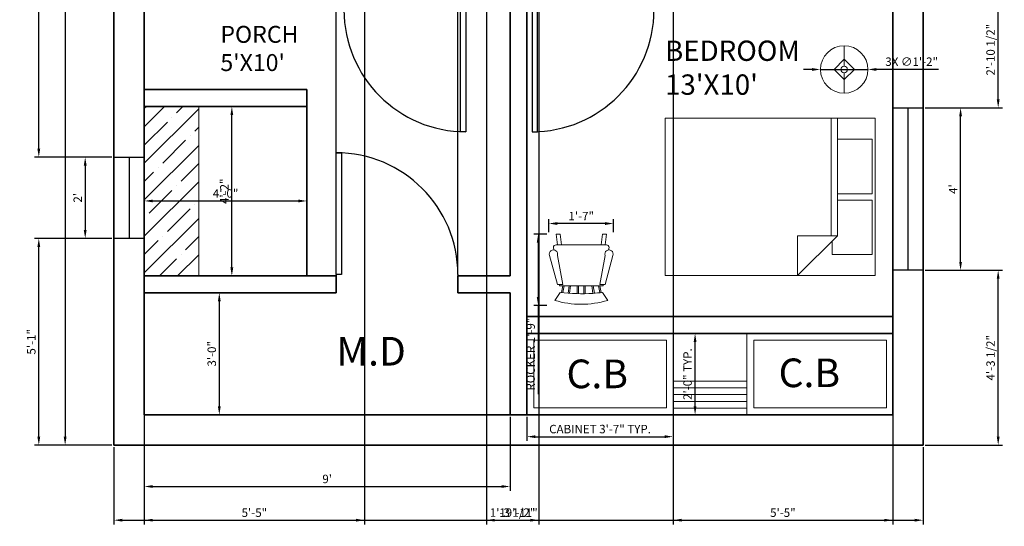
# Model space of a CAD drawing. Units: inches. Extents: x 2459 to 2755, y 1300 to 1776.
# Tile 1 of 4: x 2459 to 2750, y 1300 to 1450. Entities that reach past the tile are written whole.
import ezdxf

# ---------------------------------------------------------------- set-up
doc = ezdxf.new("R2010")
doc.units = ezdxf.units.IN
for name, color, linetype, lineweight in [('A-AREA-IDEN', 3, 'Continuous', 25), ('A-FLOR-CASE', 7, 'Continuous', 20), ('A-FURN-PATT', 8, 'Continuous', 13), ('A-WALL', 7, 'Continuous', 35), ('DIM', 4, 'Continuous', 18), ('DOOR', 20, 'Continuous', 25), ('FURNITURE', 6, 'Continuous', 18), ('TEXT', 3, 'Continuous', 25), ('WIN', 2, 'Continuous', 25)]:
    doc.layers.add(name, color=color, linetype=linetype, lineweight=lineweight)
doc.styles.get("Standard").update_dxf_attribs({"font": 'arial.ttf'})
doc.dimstyles.new('ISO-25', dxfattribs={"dimtxt": 2.5, "dimasz": 2.5, "dimexe": 1.25, "dimexo": 0.625, "dimtad": 1, "dimlunit": 3, "dimtxsty": 'Standard', "dimcen": 2.5, "dimadec": 0, "dimazin": 0, "dimtfac": 1, "dimtmove": 0, "dimatfit": 3, "dimfxl": 1, "dimarcsym": 0})

# ---------------------------------------------------------------- blocks, each defined once
blk = doc.blocks.new('*U2')
for p, q in [((0, 0), (0, -6)), ((40, 0), (40, -6))]:
    blk.add_line(p, q)
blk.add_lwpolyline([(0, 0), (0, 40), (1.75, 40), (1.75, 0)], close=True)
blk.add_arc((0, 0), 40, 0, 90)
blk = doc.blocks.new('*U5')
for p, q in [((0, 0), (0, 6)), ((40, 0), (40, 6))]:
    blk.add_line(p, q)
blk.add_lwpolyline([(0, 0), (0, -40), (1.75, -40), (1.75, 0)], close=True)
blk.add_arc((0, 0), 40, 270, 0)
blk = doc.blocks.new('*U4')
for p, q in [((-40, 0), (-40, 6)), ((0, 0), (0, 6))]:
    blk.add_line(p, q)
blk.add_lwpolyline([(0, 0), (0, -40), (-1.75, -40), (-1.75, 0)], close=True)
blk.add_arc((0, 0), 40, 180, 270)
blk = doc.blocks.new('Bed - Queen')
for p, q in [((0, -80.00003), (0, 0)), ((0, 0), (59.99999, 0)), ((59.99999, 0), (59.99999, -80.00003)), ((7.99999, -1.2), (28.79998, -1.2)), ((7.99999, -14.4), (7.99999, -1.2)), ((28.79998, -1.2), (28.79998, -14.4)), ((31.19999, -1.2), (51.99999, -1.2)), ((31.19999, -14.4), (31.19999, -1.2)), ((51.99999, -1.2), (51.99999, -16.4)), ((0, -14.4), (44.8, -14.4)), ((59.99999, -29.6), (44.8, -14.4)), ((44.8, -14.4), (44.8, -29.6)), ((44.8, -16.8), (0, -16.8)), ((51.99999, -16.4), (46.79936, -16.4)), ((44.8, -29.6), (59.99999, -29.6)), ((59.99999, -80.00003), (0, -80.00003))]:
    blk.add_line(p, q)
blk = doc.blocks.new('Lamp - Table')
for p, q in [((0, 7), (0, 1)), ((0, 3), (-3, 0)), ((3, 0), (0, 3)), ((-1, 0), (-7, 0)), ((-3, 0), (0, -3)), ((0, -3), (3, 0)), ((1, 0), (7, 0)), ((0, -1), (0, -7))]:
    blk.add_line(p, q)
for radius in [7, 1]:
    blk.add_circle((0, 0), radius)
blk = doc.blocks.new('Chair - Rocking')
for p, q in [((-8, -4.5), (-10, -1.5)), ((8, -4.5), (10, -1.5)), ((-8.23428, -6.99939), (-8.3093, -7.47958)), ((-8.23041, -7), (8.23915, -7)), ((-7.5, -4.5), (-7, -7)), ((-6.5, -7), (-7.02225, -4.43)), ((-4.5, -7), (-4.96674, -4.19951)), ((-4, -7), (-4.40532, -4.16272)), ((-1.5, -4.05012), (-1.5, -7)), ((-1, -7), (-1, -4.05012)), ((1, -7), (1, -4.04655)), ((1.5, -4.05012), (1.5, -7)), ((4, -7), (4.40187, -4.18694)), ((4.5, -7), (4.96761, -4.19437)), ((6.5, -7), (7, -4.4057)), ((7.5, -4.5), (7, -7)), ((8.31071, -7.48854), (8.23449, -7.00073)), ((-9, -7.5), (-12, -18.49999)), ((-7, -7.5), (-9, -7.5)), ((-9, -18.49999), (-7, -7.5)), ((7, -7.5), (9, -7.5)), ((9, -18.49999), (7, -7.5)), ((9, -7.5), (12, -18.49999)), ((-10.36644, -20.64523), (-10.5, -21.49999)), ((10.5, -21.49999), (10.3575, -20.58798)), ((-9, -22.49999), (-9.5, -26.49999)), ((0, -22.49999), (-9.5, -22.49999)), ((-8, -26.49999), (-7.5, -22.49999)), ((0, -22.49999), (9.5, -22.49999)), ((8, -26.49999), (7.5, -22.49999)), ((9, -22.49999), (9.5, -26.49999)), ((-9.5, -26.49999), (-8, -26.49999)), ((9.5, -26.49999), (8, -26.49999))]:
    blk.add_line(p, q)
for centre, radius, start, end in [((0, -34.08333), 34.08333, 72.93847, 107.0615), ((0, -68.25004), 64.25, 93.92211, 97.15267), ((0, -68.25004), 64.25, 82.84733, 93.92211), ((-10.5, -18.99999), 1.58114, 161.5651, 18.43495), ((10.5, -18.99999), 1.58114, 161.5651, 18.43495), ((-9.5, -21.49999), 1, 180, 270), ((9.5, -21.49999), 1, 270, 0)]:
    blk.add_arc(centre, radius, start, end)
blk = doc.blocks.new('*D19')
at = {"layer": 'Defpoints', "color": 0, "transparency": 16777216}
for p in [(2487, 1748.32), (2472.62, 1324.32), (2487, 1324.32)]:
    blk.add_point(p, dxfattribs=at)
at = {"layer": 'DIM', "color": 0, "lineweight": -2, "transparency": 16777216}
for p, q in [((2486.37, 1748.32), (2471.37, 1748.32)), ((2472.62, 1745.82), (2472.62, 1326.82)), ((2486.37, 1324.32), (2471.37, 1324.32))]:
    blk.add_line(p, q, dxfattribs=at)
at = {"layer": 'DIM', "color": 0, "transparency": 16777216}
for points in [[(2472.2, 1745.82), (2473.04, 1745.82), (2472.62, 1748.32)], [(2472.2, 1326.82), (2473.04, 1326.82), (2472.62, 1324.32)]]:
    blk.add_solid(points, dxfattribs=at)
at = {"layer": 'DIM', "color": 0, "transparency": 16777216, "insert": (2470.72, 1536.32), "char_height": 2.5, "attachment_point": 5, "rotation": 90}
blk.add_mtext('35\'-4"', dxfattribs=at)
blk = doc.blocks.new('*D24')
at = {"layer": 'Defpoints', "color": 0, "transparency": 16777216}
for p in [(2487, 1409.4), (2478.55, 1385.4), (2487, 1385.4)]:
    blk.add_point(p, dxfattribs=at)
at = {"layer": 'DIM', "color": 0, "lineweight": -2, "transparency": 16777216}
for p, q in [((2486.37, 1409.4), (2477.3, 1409.4)), ((2478.55, 1406.9), (2478.55, 1387.9)), ((2486.37, 1385.4), (2477.3, 1385.4))]:
    blk.add_line(p, q, dxfattribs=at)
at = {"layer": 'DIM', "color": 0, "transparency": 16777216}
for points in [[(2478.13, 1406.9), (2478.97, 1406.9), (2478.55, 1409.4)], [(2478.13, 1387.9), (2478.97, 1387.9), (2478.55, 1385.4)]]:
    blk.add_solid(points, dxfattribs=at)
at = {"layer": 'DIM', "color": 0, "transparency": 16777216, "insert": (2476.67, 1397.4), "char_height": 2.5, "attachment_point": 5, "rotation": 90}
blk.add_mtext("2'", dxfattribs=at)
blk = doc.blocks.new('*D25')
at = {"layer": 'Defpoints', "color": 0, "transparency": 16777216}
for p in [(2496, 1333.32), (2604, 1333.32), (2604, 1312.12)]:
    blk.add_point(p, dxfattribs=at)
at = {"layer": 'DIM', "color": 0, "lineweight": -2, "transparency": 16777216}
for p, q in [((2496, 1332.69), (2496, 1310.87)), ((2604, 1332.69), (2604, 1310.87)), ((2498.5, 1312.12), (2601.5, 1312.12))]:
    blk.add_line(p, q, dxfattribs=at)
at = {"layer": 'DIM', "color": 0, "transparency": 16777216}
for points in [[(2498.5, 1312.54), (2498.5, 1311.71), (2496, 1312.12)], [(2601.5, 1312.54), (2601.5, 1311.71), (2604, 1312.12)]]:
    blk.add_solid(points, dxfattribs=at)
at = {"layer": 'DIM', "color": 0, "transparency": 16777216, "insert": (2550, 1314.03), "char_height": 2.5, "attachment_point": 5}
blk.add_mtext("9'", dxfattribs=at)
blk = doc.blocks.new('*D26')
at = {"layer": 'Defpoints', "color": 0, "transparency": 16777216}
for p in [(2726, 1423.98), (2737.04, 1423.98), (2726, 1375.98)]:
    blk.add_point(p, dxfattribs=at)
at = {"layer": 'DIM', "color": 0, "lineweight": -2, "transparency": 16777216}
for p, q in [((2726.62, 1423.98), (2738.29, 1423.98)), ((2737.04, 1378.48), (2737.04, 1421.48)), ((2726.62, 1375.98), (2738.29, 1375.98))]:
    blk.add_line(p, q, dxfattribs=at)
at = {"layer": 'DIM', "color": 0, "transparency": 16777216}
for points in [[(2736.63, 1421.48), (2737.46, 1421.48), (2737.04, 1423.98)], [(2736.63, 1378.48), (2737.46, 1378.48), (2737.04, 1375.98)]]:
    blk.add_solid(points, dxfattribs=at)
at = {"layer": 'DIM', "color": 0, "transparency": 16777216, "insert": (2735.17, 1399.98), "char_height": 2.5, "attachment_point": 5, "rotation": 90}
blk.add_mtext("4'", dxfattribs=at)
blk = doc.blocks.new('WIN-48IN')
blk.add_line((4.5, 48), (4.5, 0))
blk.add_lwpolyline([(0, 48), (9, 48), (9, 0), (0, 0)], close=True)
blk = doc.blocks.new('WIN-24IN')
blk.add_line((4.5, 24), (4.5, 0))
blk.add_lwpolyline([(0, 24), (9, 24), (9, 0), (0, 0)], close=True)
blk = doc.blocks.new('CABINET-43X24IN')
for points in [[(0, 24), (43.17, 24), (43.17, 0), (0, 0)], [(2, 22), (41.17, 22), (41.17, 2), (2, 2)]]:
    blk.add_lwpolyline(points, close=True)
blk = doc.blocks.new('*D39')
at = {"layer": 'Defpoints', "color": 0, "transparency": 16777216}
for p in [(2615.48, 1386.64), (2612.32, 1365.55), (2615.48, 1365.55)]:
    blk.add_point(p, dxfattribs=at)
at = {"layer": 'DIM', "color": 0, "lineweight": -2, "transparency": 16777216}
for p, q in [((2614.86, 1386.64), (2611.07, 1386.64)), ((2612.32, 1384.14), (2612.32, 1368.05)), ((2614.86, 1365.55), (2611.07, 1365.55)), ((2612.32, 1365.55), (2612.32, 1339.37))]:
    blk.add_line(p, q, dxfattribs=at)
at = {"layer": 'DIM', "color": 0, "transparency": 16777216}
for points in [[(2611.9, 1384.14), (2612.73, 1384.14), (2612.32, 1386.64)], [(2611.9, 1368.05), (2612.73, 1368.05), (2612.32, 1365.55)]]:
    blk.add_solid(points, dxfattribs=at)
at = {"layer": 'DIM', "color": 0, "transparency": 16777216, "insert": (2610.4, 1351.21), "char_height": 2.5, "attachment_point": 5, "rotation": 90}
blk.add_mtext('ROCKER 1\'-9"', dxfattribs=at)
blk = doc.blocks.new('*D40')
at = {"layer": 'Defpoints', "color": 0, "transparency": 16777216}
for p in [(2615.48, 1389.8), (2615.48, 1386.64), (2634.57, 1386.64)]:
    blk.add_point(p, dxfattribs=at)
at = {"layer": 'DIM', "color": 0, "lineweight": -2, "transparency": 16777216}
for p, q in [((2615.48, 1387.26), (2615.48, 1391.05)), ((2634.57, 1387.26), (2634.57, 1391.05)), ((2632.07, 1389.8), (2617.98, 1389.8))]:
    blk.add_line(p, q, dxfattribs=at)
at = {"layer": 'DIM', "color": 0, "transparency": 16777216}
for points in [[(2617.98, 1390.22), (2617.98, 1389.38), (2615.48, 1389.8)], [(2632.07, 1390.22), (2632.07, 1389.38), (2634.57, 1389.8)]]:
    blk.add_solid(points, dxfattribs=at)
at = {"layer": 'DIM', "color": 0, "transparency": 16777216, "insert": (2625.02, 1391.68), "char_height": 2.5, "attachment_point": 5}
blk.add_mtext('1\'-7"', dxfattribs=at)
blk = doc.blocks.new('*D43')
at = {"layer": 'Defpoints', "color": 0, "transparency": 16777216}
for p in [(2609, 1333.32), (2652.16, 1333.32), (2652.16, 1326.84)]:
    blk.add_point(p, dxfattribs=at)
at = {"layer": 'DIM', "color": 0, "lineweight": -2, "transparency": 16777216}
for p, q in [((2609, 1332.69), (2609, 1325.59)), ((2652.16, 1332.69), (2652.16, 1325.59)), ((2611.5, 1326.84), (2649.66, 1326.84))]:
    blk.add_line(p, q, dxfattribs=at)
at = {"layer": 'DIM', "color": 0, "transparency": 16777216}
for points in [[(2611.5, 1327.26), (2611.5, 1326.43), (2609, 1326.84)], [(2649.66, 1327.26), (2649.66, 1326.43), (2652.16, 1326.84)]]:
    blk.add_solid(points, dxfattribs=at)
at = {"layer": 'DIM', "color": 0, "transparency": 16777216, "insert": (2630.58, 1328.76), "char_height": 2.5, "attachment_point": 5}
blk.add_mtext('CABINET 3\'-7" TYP.', dxfattribs=at)
blk = doc.blocks.new('*D44')
at = {"layer": 'Defpoints', "color": 0, "transparency": 16777216}
for p in [(2652.16, 1357.32), (2658.64, 1357.32), (2652.16, 1333.32)]:
    blk.add_point(p, dxfattribs=at)
at = {"layer": 'DIM', "color": 0, "lineweight": -2, "transparency": 16777216}
for p, q in [((2652.79, 1357.32), (2659.89, 1357.32)), ((2658.64, 1335.82), (2658.64, 1354.82)), ((2652.79, 1333.32), (2659.89, 1333.32))]:
    blk.add_line(p, q, dxfattribs=at)
at = {"layer": 'DIM', "color": 0, "transparency": 16777216}
for points in [[(2658.22, 1354.82), (2659.06, 1354.82), (2658.64, 1357.32)], [(2658.22, 1335.82), (2659.06, 1335.82), (2658.64, 1333.32)]]:
    blk.add_solid(points, dxfattribs=at)
at = {"layer": 'DIM', "color": 0, "transparency": 16777216, "insert": (2656.74, 1345.32), "char_height": 2.5, "attachment_point": 5, "rotation": 90}
blk.add_mtext('2\'-0" TYP.', dxfattribs=at)
blk = doc.blocks.new('*D57')
at = {"layer": 'Defpoints', "color": 0, "transparency": 16777216}
for p in [(2487, 1324.32), (2726, 1324.32), (2726, 1302.17)]:
    blk.add_point(p, dxfattribs=at)
at = {"layer": 'DIM', "color": 0, "lineweight": -2, "transparency": 16777216}
for p, q in [((2487, 1323.69), (2487, 1300.92)), ((2726, 1323.69), (2726, 1300.92)), ((2489.5, 1302.17), (2723.5, 1302.17))]:
    blk.add_line(p, q, dxfattribs=at)
at = {"layer": 'DIM', "color": 0, "transparency": 16777216}
for points in [[(2489.5, 1302.58), (2489.5, 1301.75), (2487, 1302.17)], [(2723.5, 1302.58), (2723.5, 1301.75), (2726, 1302.17)]]:
    blk.add_solid(points, dxfattribs=at)
at = {"layer": 'DIM', "color": 0, "transparency": 16777216, "insert": (2606.5, 1304.07), "char_height": 2.5, "attachment_point": 5}
blk.add_mtext('19\'-11"', dxfattribs=at)
blk = doc.blocks.new('*D62')
at = {"layer": 'Defpoints', "color": 0, "transparency": 16777216}
for p in [(2464.85, 1385.4), (2487, 1385.4), (2487, 1324.32)]:
    blk.add_point(p, dxfattribs=at)
at = {"layer": 'DIM', "color": 0, "lineweight": -2, "transparency": 16777216}
for p, q in [((2486.37, 1385.4), (2463.6, 1385.4)), ((2464.85, 1326.82), (2464.85, 1382.9)), ((2486.37, 1324.32), (2463.6, 1324.32))]:
    blk.add_line(p, q, dxfattribs=at)
at = {"layer": 'DIM', "color": 0, "transparency": 16777216}
for points in [[(2464.43, 1382.9), (2465.26, 1382.9), (2464.85, 1385.4)], [(2464.43, 1326.82), (2465.26, 1326.82), (2464.85, 1324.32)]]:
    blk.add_solid(points, dxfattribs=at)
at = {"layer": 'DIM', "color": 0, "transparency": 16777216, "insert": (2462.95, 1354.86), "char_height": 2.5, "attachment_point": 5, "rotation": 90}
blk.add_mtext('5\'-1"', dxfattribs=at)
blk = doc.blocks.new('*D63')
at = {"layer": 'Defpoints', "color": 0, "transparency": 16777216}
for p in [(2464.85, 1517.93), (2487, 1517.93), (2487, 1409.4)]:
    blk.add_point(p, dxfattribs=at)
at = {"layer": 'DIM', "color": 0, "lineweight": -2, "transparency": 16777216}
for p, q in [((2486.37, 1517.93), (2463.6, 1517.93)), ((2464.85, 1411.9), (2464.85, 1515.43)), ((2486.37, 1409.4), (2463.6, 1409.4))]:
    blk.add_line(p, q, dxfattribs=at)
at = {"layer": 'DIM', "color": 0, "transparency": 16777216}
for points in [[(2464.43, 1515.43), (2465.26, 1515.43), (2464.85, 1517.93)], [(2464.43, 1411.9), (2465.26, 1411.9), (2464.85, 1409.4)]]:
    blk.add_solid(points, dxfattribs=at)
at = {"layer": 'DIM', "color": 0, "transparency": 16777216, "insert": (2462.93, 1463.67), "char_height": 2.5, "attachment_point": 5, "rotation": 90}
blk.add_mtext('9\'-0 1/2"', dxfattribs=at)
blk = doc.blocks.new('*D65')
at = {"layer": 'Defpoints', "color": 0, "transparency": 16777216}
for p in [(2726, 1375.98), (2748.15, 1375.98), (2726, 1324.32)]:
    blk.add_point(p, dxfattribs=at)
at = {"layer": 'DIM', "color": 0, "lineweight": -2, "transparency": 16777216}
for p, q in [((2726.62, 1375.98), (2749.4, 1375.98)), ((2748.15, 1326.82), (2748.15, 1373.48)), ((2726.62, 1324.32), (2749.4, 1324.32))]:
    blk.add_line(p, q, dxfattribs=at)
at = {"layer": 'DIM', "color": 0, "transparency": 16777216}
for points in [[(2747.73, 1373.48), (2748.56, 1373.48), (2748.15, 1375.98)], [(2747.73, 1326.82), (2748.56, 1326.82), (2748.15, 1324.32)]]:
    blk.add_solid(points, dxfattribs=at)
at = {"layer": 'DIM', "color": 0, "transparency": 16777216, "insert": (2746.23, 1350.15), "char_height": 2.5, "attachment_point": 5, "rotation": 90}
blk.add_mtext('4\'-3 1/2"', dxfattribs=at)
blk = doc.blocks.new('*D66')
at = {"layer": 'Defpoints', "color": 0, "transparency": 16777216}
for p in [(2717, 1458.32), (2748.15, 1458.32), (2726, 1423.98)]:
    blk.add_point(p, dxfattribs=at)
at = {"layer": 'DIM', "color": 0, "lineweight": -2, "transparency": 16777216}
for p, q in [((2717.62, 1458.32), (2749.4, 1458.32)), ((2748.15, 1426.48), (2748.15, 1455.82)), ((2726.62, 1423.98), (2749.4, 1423.98))]:
    blk.add_line(p, q, dxfattribs=at)
at = {"layer": 'DIM', "color": 0, "transparency": 16777216}
for points in [[(2747.73, 1455.82), (2748.56, 1455.82), (2748.15, 1458.32)], [(2747.73, 1426.48), (2748.56, 1426.48), (2748.15, 1423.98)]]:
    blk.add_solid(points, dxfattribs=at)
at = {"layer": 'DIM', "color": 0, "transparency": 16777216, "insert": (2746.23, 1441.15), "char_height": 2.5, "attachment_point": 5, "rotation": 90}
blk.add_mtext('2\'-10 1/2"', dxfattribs=at)
blk = doc.blocks.new('*D70')
at = {"layer": 'Defpoints', "color": 0, "transparency": 16777216}
for p in [(2588.61, 1770.47), (2552.61, 1374.32), (2588.61, 1374.32)]:
    blk.add_point(p, dxfattribs=at)
at = {"layer": 'DIM', "color": 0, "lineweight": -2, "transparency": 16777216}
for p, q in [((2552.61, 1374.94), (2552.61, 1771.72)), ((2588.61, 1374.94), (2588.61, 1771.72)), ((2555.11, 1770.47), (2586.11, 1770.47))]:
    blk.add_line(p, q, dxfattribs=at)
at = {"layer": 'DIM', "color": 0, "transparency": 16777216}
for points in [[(2555.11, 1770.88), (2555.11, 1770.05), (2552.61, 1770.47)], [(2586.11, 1770.88), (2586.11, 1770.05), (2588.61, 1770.47)]]:
    blk.add_solid(points, dxfattribs=at)
at = {"layer": 'DIM', "color": 0, "transparency": 16777216, "insert": (2570.61, 1772.37), "char_height": 2.5, "attachment_point": 5}
blk.add_mtext('3\'-0"', dxfattribs=at)
blk = doc.blocks.new('*D72')
at = {"layer": 'Defpoints', "color": 0, "transparency": 16777216}
for p in [(2652.14, 1614.32), (2717, 1614.32), (2717, 1302.17)]:
    blk.add_point(p, dxfattribs=at)
at = {"layer": 'DIM', "color": 0, "lineweight": -2, "transparency": 16777216}
for p, q in [((2652.14, 1613.69), (2652.14, 1300.92)), ((2717, 1613.69), (2717, 1300.92)), ((2654.64, 1302.17), (2714.5, 1302.17))]:
    blk.add_line(p, q, dxfattribs=at)
at = {"layer": 'DIM', "color": 0, "transparency": 16777216}
for points in [[(2654.64, 1302.58), (2654.64, 1301.75), (2652.14, 1302.17)], [(2714.5, 1302.58), (2714.5, 1301.75), (2717, 1302.17)]]:
    blk.add_solid(points, dxfattribs=at)
at = {"layer": 'DIM', "color": 0, "transparency": 16777216, "insert": (2684.57, 1304.06), "char_height": 2.5, "attachment_point": 5}
blk.add_mtext('5\'-5"', dxfattribs=at)
blk = doc.blocks.new('*D75')
at = {"layer": 'Defpoints', "color": 0, "transparency": 16777216}
for p in [(2496, 1614.32), (2561, 1614.32), (2561, 1302.17)]:
    blk.add_point(p, dxfattribs=at)
at = {"layer": 'DIM', "color": 0, "lineweight": -2, "transparency": 16777216}
for p, q in [((2496, 1613.69), (2496, 1300.92)), ((2561, 1613.69), (2561, 1300.92)), ((2498.5, 1302.17), (2558.5, 1302.17))]:
    blk.add_line(p, q, dxfattribs=at)
at = {"layer": 'DIM', "color": 0, "transparency": 16777216}
for points in [[(2498.5, 1302.58), (2498.5, 1301.75), (2496, 1302.17)], [(2558.5, 1302.58), (2558.5, 1301.75), (2561, 1302.17)]]:
    blk.add_solid(points, dxfattribs=at)
at = {"layer": 'DIM', "color": 0, "transparency": 16777216, "insert": (2528.5, 1304.06), "char_height": 2.5, "attachment_point": 5}
blk.add_mtext('5\'-5"', dxfattribs=at)
blk = doc.blocks.new('*D76')
at = {"layer": 'Defpoints', "color": 0, "transparency": 16777216}
for p in [(2597, 1614.32), (2612.48, 1614.32), (2612.48, 1302.17)]:
    blk.add_point(p, dxfattribs=at)
at = {"layer": 'DIM', "color": 0, "lineweight": -2, "transparency": 16777216}
for p, q in [((2597, 1613.69), (2597, 1300.92)), ((2612.48, 1613.69), (2612.48, 1300.92)), ((2599.5, 1302.17), (2609.98, 1302.17))]:
    blk.add_line(p, q, dxfattribs=at)
at = {"layer": 'DIM', "color": 0, "transparency": 16777216}
for points in [[(2599.5, 1302.58), (2599.5, 1301.75), (2597, 1302.17)], [(2609.98, 1302.58), (2609.98, 1301.75), (2612.48, 1302.17)]]:
    blk.add_solid(points, dxfattribs=at)
at = {"layer": 'DIM', "color": 0, "transparency": 16777216, "insert": (2604.74, 1304.09), "char_height": 2.5, "attachment_point": 5}
blk.add_mtext('1\'-3 1/2"', dxfattribs=at)
blk = doc.blocks.new('*D79')
at = {"layer": 'Defpoints', "color": 0, "transparency": 16777216}
for p in [(2604, 1770.47), (2588.61, 1374.32), (2604, 1374.32)]:
    blk.add_point(p, dxfattribs=at)
at = {"layer": 'DIM', "color": 0, "lineweight": -2, "transparency": 16777216}
for p, q in [((2588.61, 1374.94), (2588.61, 1771.72)), ((2604, 1374.94), (2604, 1771.72)), ((2591.11, 1770.47), (2601.5, 1770.47))]:
    blk.add_line(p, q, dxfattribs=at)
at = {"layer": 'DIM', "color": 0, "transparency": 16777216}
for points in [[(2591.11, 1770.88), (2591.11, 1770.05), (2588.61, 1770.47)], [(2601.5, 1770.88), (2601.5, 1770.05), (2604, 1770.47)]]:
    blk.add_solid(points, dxfattribs=at)
at = {"layer": 'DIM', "color": 0, "transparency": 16777216, "insert": (2596.3, 1772.39), "char_height": 2.5, "attachment_point": 5}
blk.add_mtext('1\'-3 1/2"', dxfattribs=at)
blk = doc.blocks.new('*D80')
at = {"layer": 'Defpoints', "color": 0, "transparency": 16777216}
for p in [(2496, 1369.32), (2496, 1333.32), (2518.15, 1333.32)]:
    blk.add_point(p, dxfattribs=at)
at = {"layer": 'DIM', "color": 0, "lineweight": -2, "transparency": 16777216}
for p, q in [((2496.62, 1369.32), (2519.4, 1369.32)), ((2518.15, 1366.82), (2518.15, 1335.82)), ((2496.62, 1333.32), (2519.4, 1333.32))]:
    blk.add_line(p, q, dxfattribs=at)
at = {"layer": 'DIM', "color": 0, "transparency": 16777216}
for points in [[(2517.73, 1366.82), (2518.56, 1366.82), (2518.15, 1369.32)], [(2517.73, 1335.82), (2518.56, 1335.82), (2518.15, 1333.32)]]:
    blk.add_solid(points, dxfattribs=at)
at = {"layer": 'DIM', "color": 0, "transparency": 16777216, "insert": (2516.24, 1351.32), "char_height": 2.5, "attachment_point": 5, "rotation": 90}
blk.add_mtext('3\'-0"', dxfattribs=at)
blk = doc.blocks.new('*D81')
at = {"layer": 'Defpoints', "color": 0, "transparency": 16777216}
for p in [(2544, 1396.47), (2496, 1374.32), (2544, 1374.32)]:
    blk.add_point(p, dxfattribs=at)
at = {"layer": 'DIM', "color": 0, "lineweight": -2, "transparency": 16777216}
for p, q in [((2496, 1374.94), (2496, 1397.72)), ((2498.5, 1396.47), (2541.5, 1396.47)), ((2544, 1374.94), (2544, 1397.72))]:
    blk.add_line(p, q, dxfattribs=at)
at = {"layer": 'DIM', "color": 0, "transparency": 16777216}
for points in [[(2498.5, 1396.88), (2498.5, 1396.05), (2496, 1396.47)], [(2541.5, 1396.88), (2541.5, 1396.05), (2544, 1396.47)]]:
    blk.add_solid(points, dxfattribs=at)
at = {"layer": 'DIM', "color": 0, "transparency": 16777216, "insert": (2520, 1398.37), "char_height": 2.5, "attachment_point": 5}
blk.add_mtext('4\'-0"', dxfattribs=at)
blk = doc.blocks.new('*D82')
at = {"layer": 'Defpoints', "color": 0, "transparency": 16777216}
for p in [(2521.85, 1424.36), (2544, 1424.36), (2544, 1374.32)]:
    blk.add_point(p, dxfattribs=at)
at = {"layer": 'DIM', "color": 0, "lineweight": -2, "transparency": 16777216}
for p, q in [((2543.37, 1424.36), (2520.6, 1424.36)), ((2521.85, 1376.82), (2521.85, 1421.86)), ((2543.37, 1374.32), (2520.6, 1374.32))]:
    blk.add_line(p, q, dxfattribs=at)
at = {"layer": 'DIM', "color": 0, "transparency": 16777216}
for points in [[(2521.43, 1421.86), (2522.26, 1421.86), (2521.85, 1424.36)], [(2521.43, 1376.82), (2522.26, 1376.82), (2521.85, 1374.32)]]:
    blk.add_solid(points, dxfattribs=at)
at = {"layer": 'DIM', "color": 0, "transparency": 16777216, "insert": (2519.97, 1399.34), "char_height": 2.5, "attachment_point": 5, "rotation": 90}
blk.add_mtext('4\'-2"', dxfattribs=at)
blk = doc.blocks.new('*D84')
at = {"layer": 'Defpoints', "color": 0, "transparency": 16777216}
for p in [(2695.67, 1435.32), (2709.67, 1435.32)]:
    blk.add_point(p, dxfattribs=at)
at = {"layer": 'DIM', "color": 0, "lineweight": -2, "transparency": 16777216}
for p, q in [((2693.17, 1435.32), (2690.67, 1435.32)), ((2695.67, 1435.32), (2709.67, 1435.32)), ((2730.53, 1435.32), (2712.17, 1435.32))]:
    blk.add_line(p, q, dxfattribs=at)
at = {"layer": 'DIM', "color": 0, "transparency": 16777216}
for points in [[(2693.17, 1435.73), (2693.17, 1434.9), (2695.67, 1435.32)], [(2712.17, 1435.73), (2712.17, 1434.9), (2709.67, 1435.32)]]:
    blk.add_solid(points, dxfattribs=at)
at = {"layer": 'DIM', "color": 0, "transparency": 16777216, "insert": (2722.6, 1437.29), "char_height": 2.5, "attachment_point": 5, "rotation": 359.9971}
blk.add_mtext('3X ∅1\'-2"', dxfattribs=at)

msp = doc.modelspace()

# ---------------------------------------------------------------- hatches: boundary and pattern name
at = {"layer": 'A-FURN-PATT', "transparency": 33554521}
h = msp.add_hatch(dxfattribs=at)
h.set_pattern_fill('ANSI35', color=256, scale=1.2)
h.paths.add_polyline_path([(2512.06, 1424.362), (2495.997, 1424.362), (2495.997, 1374.317), (2512.06, 1374.317)])

# ---------------------------------------------------------------- linework, layer by layer
at = {"layer": 'A-FLOR-CASE'}
for p, q in [((2652.164, 1343.273), (2673.972, 1343.273)), ((2652.164, 1333.317), (2652.164, 1343.273)), ((2652.164, 1341.273), (2673.972, 1341.273)), ((2673.972, 1343.273), (2673.972, 1333.317)), ((2652.164, 1339.273), (2673.972, 1339.273)), ((2652.164, 1337.273), (2673.972, 1337.273)), ((2652.164, 1335.273), (2673.972, 1335.273)), ((2673.972, 1333.317), (2652.164, 1333.317))]:
    msp.add_line(p, q, dxfattribs=at)
at = {"layer": 'A-WALL'}
for p, q in [((2486.997, 1324.317), (2486.997, 1748.317)), ((2725.997, 1324.317), (2725.997, 1748.317)), ((2716.997, 1333.317), (2716.997, 1739.317)), ((2495.997, 1333.317), (2495.997, 1614.317)), ((2495.997, 1333.317), (2495.997, 1488.317)), ((2603.997, 1374.317), (2603.997, 1453.317)), ((2608.997, 1362.317), (2608.997, 1453.317)), ((2495.997, 1429.362), (2543.997, 1429.362)), ((2543.997, 1374.317), (2543.997, 1429.362)), ((2495.997, 1374.317), (2495.997, 1424.362)), ((2495.997, 1424.362), (2543.997, 1424.362)), ((2552.609, 1374.317), (2495.997, 1374.317)), ((2603.997, 1374.317), (2588.609, 1374.317)), ((2552.609, 1369.317), (2495.997, 1369.317)), ((2603.997, 1369.317), (2588.609, 1369.317)), ((2603.997, 1333.317), (2603.997, 1369.317)), ((2608.997, 1362.317), (2716.997, 1362.317)), ((2608.997, 1357.317), (2608.997, 1362.317)), ((2608.997, 1357.317), (2716.997, 1357.317)), ((2608.997, 1333.317), (2608.997, 1357.317)), ((2495.997, 1333.317), (2716.997, 1333.317)), ((2486.997, 1324.317), (2725.997, 1324.317))]:
    msp.add_line(p, q, dxfattribs=at)
for points in [[(2552.609, 1369.317), (2552.609, 1374.317)], [(2588.609, 1374.317), (2588.609, 1369.317)]]:
    msp.add_lwpolyline(points, dxfattribs=at)
at = {"layer": 'FURNITURE'}
msp.add_lwpolyline([(2495.997, 1424.362), (2512.06, 1424.362), (2512.06, 1374.317), (2495.997, 1374.317)], close=True, dxfattribs=at)

# ---------------------------------------------------------------- block references
at = {"layer": 'A-FLOR-CASE'}
for p in [(2608.997, 1333.317), (2673.972, 1333.317)]:
    msp.add_blockref('CABINET-43X24IN', p, dxfattribs=at)
at = {"layer": 'DOOR', "xscale": 0.9, "yscale": 0.9, "zscale": 0.9}
for name, p in [('*U4', (2590.966, 1452.917)), ('*U5', (2610.511, 1452.917)), ('*U2', (2552.609, 1374.717)), ('*U2', (2552.609, 1374.717))]:
    msp.add_blockref(name, p, dxfattribs=at)
at = {"layer": 'FURNITURE'}
msp.add_blockref('Lamp - Table', (2702.674, 1435.317), dxfattribs=at)
for name, p, xscale, yscale, zscale, rotation in [('Bed - Queen', (2711.827, 1420.944), 0.775599459013597, 0.775599459013597, 0.775599459013597, 270), ('Chair - Rocking', (2625.024, 1365.94), 0.7810468391343605, 0.7810468391343605, 0.7810468391343605, 180)]:
    msp.add_blockref(name, p, dxfattribs=dict(at, xscale=xscale, yscale=yscale, zscale=zscale, rotation=rotation))
at = {"layer": 'WIN'}
for name, p in [('WIN-48IN', (2716.997, 1375.985)), ('WIN-24IN', (2486.997, 1385.402))]:
    msp.add_blockref(name, p, dxfattribs=at)

# ---------------------------------------------------------------- texts
at = {"layer": 'A-AREA-IDEN', "attachment_point": 1}
for s, insert, char_height in [("{PORCH\\P5'X10'}", (2518.467, 1448.184), 5), ("{BEDROOM\\P13'X10'}", (2649.779, 1443.844), 6)]:
    msp.add_mtext_dynamic_manual_height_columns(s, width=133.04104, gutter_width=21.155, heights=[0], dxfattribs=dict(at, insert=insert, char_height=char_height))
at = {"layer": 'TEXT', "char_height": 8.4618, "attachment_point": 1}
for s, insert in [('{M.D}', (2552.715, 1356.301)), ('{C.B}', (2620.67, 1349.619)), ('{C.B}', (2683.306, 1349.928))]:
    msp.add_mtext_dynamic_manual_height_columns(s, width=133.04104, gutter_width=21.155, heights=[0], dxfattribs=dict(at, insert=insert))

# ---------------------------------------------------------------- dimensions: what is measured, and where the dimension line sits
at = {"layer": 'DIM'}
for base, p1, p2, override, picture, middle in [((2588.609, 1770.467), (2552.609, 1374.317), (2588.609, 1374.317), {"dimdec": 1, "dimlfac": 1, "dimrnd": 0, "dimzin": 1, "dimdsep": 46, "dimlunit": 4, "dimfrac": 2}, '*D70', (2570.609, 1772.369)), ((2603.997, 1770.467), (2588.609, 1374.317), (2603.997, 1374.317), {"dimdec": 1, "dimlfac": 1, "dimrnd": 0, "dimzin": 1, "dimdsep": 46, "dimlunit": 4, "dimfrac": 2}, '*D79', (2596.303, 1772.386)), ((2560.996, 1302.167), (2495.997, 1614.317), (2560.996, 1614.317), {"dimdec": 1, "dimlfac": 1, "dimrnd": 0, "dimzin": 1, "dimdsep": 46, "dimlunit": 4, "dimfrac": 2}, '*D75', (2528.496, 1304.063)), ((2612.476, 1302.167), (2596.996, 1614.317), (2612.476, 1614.317), {"dimdec": 1, "dimlfac": 1, "dimrnd": 0, "dimzin": 1, "dimdsep": 46, "dimlunit": 4, "dimfrac": 2}, '*D76', (2604.736, 1304.086)), ((2716.997, 1302.167), (2652.141, 1614.317), (2716.997, 1614.317), {"dimdec": 1, "dimlfac": 1, "dimrnd": 0, "dimzin": 1, "dimdsep": 46, "dimlunit": 4, "dimfrac": 2}, '*D72', (2684.569, 1304.063)), ((2543.997, 1396.467), (2495.997, 1374.317), (2543.997, 1374.317), {"dimdec": 1, "dimlfac": 1, "dimrnd": 0, "dimzin": 1, "dimdsep": 46, "dimlunit": 4, "dimfrac": 2}, '*D81', (2519.997, 1398.369)), ((2603.997, 1312.124), (2495.997, 1333.317), (2603.997, 1333.317), {"dimclrd": 0, "dimclre": 0, "dimclrt": 0}, '*D25', (2549.997, 1314.025)), ((2725.997, 1302.167), (2486.997, 1324.317), (2725.997, 1324.317), {"dimdec": 1, "dimlfac": 1, "dimrnd": 0, "dimzin": 1, "dimdsep": 46, "dimlunit": 4, "dimfrac": 2}, '*D57', (2606.497, 1304.069))]:
    dim = msp.add_linear_dim(base=base, p1=p1, p2=p2, dimstyle='ISO-25', override=override, dxfattribs=at)
    dim.commit()
    dim.dimension.update_dxf_attribs({"geometry": picture, "text_midpoint": middle})
for base, p1, p2, angle, override, picture, middle in [((2472.619, 1324.317), (2486.997, 1748.317), (2486.997, 1324.317), 90, {"dimclrd": 0, "dimclre": 0, "dimclrt": 0}, '*D19', (2470.717, 1536.317)), ((2464.847, 1517.934), (2486.997, 1409.402), (2486.997, 1517.934), 90, {"dimdec": 1, "dimlfac": 1, "dimrnd": 0, "dimzin": 1, "dimdsep": 46, "dimlunit": 4, "dimfrac": 2}, '*D63', (2462.929, 1463.668)), ((2748.147, 1458.317), (2725.997, 1423.984), (2716.997, 1458.317), 90, {"dimdec": 1, "dimlfac": 1, "dimrnd": 0, "dimzin": 1, "dimdsep": 46, "dimlunit": 4, "dimfrac": 2}, '*D66', (2746.229, 1441.151)), ((2521.847, 1424.362), (2543.997, 1374.317), (2543.997, 1424.362), 90, {"dimdec": 1, "dimlfac": 1, "dimrnd": 0, "dimzin": 1, "dimdsep": 46, "dimlunit": 4, "dimfrac": 2}, '*D82', (2519.967, 1399.339)), ((2737.042, 1423.984), (2725.997, 1375.984), (2725.997, 1423.984), 90, {"dimclrd": 0, "dimclre": 0, "dimclrt": 0}, '*D26', (2735.167, 1399.984)), ((2478.551, 1385.402), (2486.997, 1409.402), (2486.997, 1385.402), 90, {"dimclrd": 0, "dimclre": 0, "dimclrt": 0}, '*D24', (2476.671, 1397.402)), ((2615.481, 1389.801), (2634.566, 1386.638), (2615.481, 1386.638), 180, {"dimdec": 1, "dimlfac": 1, "dimrnd": 0, "dimzin": 1, "dimdsep": 46, "dimlunit": 4, "dimfrac": 2}, '*D40', (2625.024, 1391.681)), ((2464.847, 1385.402), (2486.997, 1324.317), (2486.997, 1385.402), 90, {"dimdec": 1, "dimlfac": 1, "dimrnd": 0, "dimzin": 1, "dimdsep": 46, "dimlunit": 4, "dimfrac": 2}, '*D62', (2462.945, 1354.86)), ((2748.147, 1375.984), (2725.997, 1324.317), (2725.997, 1375.984), 90, {"dimdec": 1, "dimlfac": 1, "dimrnd": 0, "dimzin": 1, "dimdsep": 46, "dimlunit": 4, "dimfrac": 2}, '*D65', (2746.228, 1350.151)), ((2518.147, 1333.317), (2495.997, 1369.317), (2495.997, 1333.317), 270, {"dimdec": 1, "dimlfac": 1, "dimrnd": 0, "dimzin": 1, "dimdsep": 46, "dimlunit": 4, "dimfrac": 2}, '*D80', (2516.245, 1351.317))]:
    dim = msp.add_linear_dim(base=base, p1=p1, p2=p2, angle=angle, dimstyle='ISO-25', override=override, dxfattribs=at)
    dim.commit()
    dim.dimension.update_dxf_attribs({"geometry": picture, "text_midpoint": middle})
dim = msp.add_diameter_dim_2p(p1=(2695.674, 1435.318), p2=(2709.674, 1435.317), text='3X <>', dimstyle='ISO-25', override={"dimdec": 1, "dimlfac": 1, "dimrnd": 0, "dimzin": 1, "dimdsep": 46, "dimlunit": 4, "dimfrac": 2}, dxfattribs=at)
dim.commit()
dim.dimension.update_dxf_attribs({"geometry": '*D84', "text_midpoint": (2722.6, 1435.316), "dimtype": 163})
for base, p1, p2, angle, text, picture, middle in [((2612.318, 1365.549), (2615.481, 1386.638), (2615.481, 1365.549), 270, 'ROCKER <>', '*D39', (2610.399, 1351.21)), ((2658.639, 1357.317), (2652.164, 1333.317), (2652.164, 1357.317), 90, '<> TYP.', '*D44', (2656.737, 1345.317))]:
    dim = msp.add_linear_dim(base=base, p1=p1, p2=p2, angle=angle, text=text, dimstyle='ISO-25', override={"dimdec": 1, "dimlfac": 1, "dimrnd": 0, "dimzin": 1, "dimdsep": 46, "dimlunit": 4, "dimfrac": 2}, dxfattribs=at)
    dim.commit()
    dim.dimension.update_dxf_attribs({"geometry": picture, "text_midpoint": middle})
dim = msp.add_linear_dim(base=(2652.164, 1326.842), p1=(2608.997, 1333.317), p2=(2652.164, 1333.317), text='CABINET <> TYP.', dimstyle='ISO-25', override={"dimdec": 1, "dimlfac": 1, "dimrnd": 0, "dimzin": 1, "dimdsep": 46, "dimlunit": 4, "dimfrac": 2}, dxfattribs=at)
dim.commit()
dim.dimension.update_dxf_attribs({"geometry": '*D43', "text_midpoint": (2630.58, 1328.761)})

doc.saveas('drawing.dxf')
